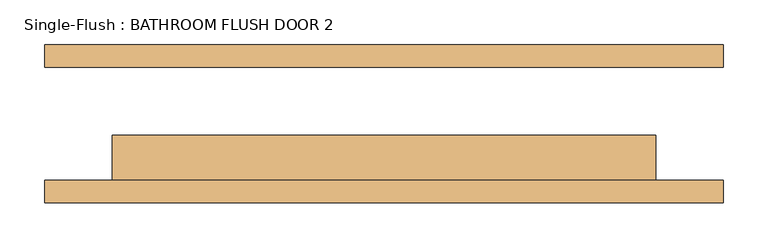
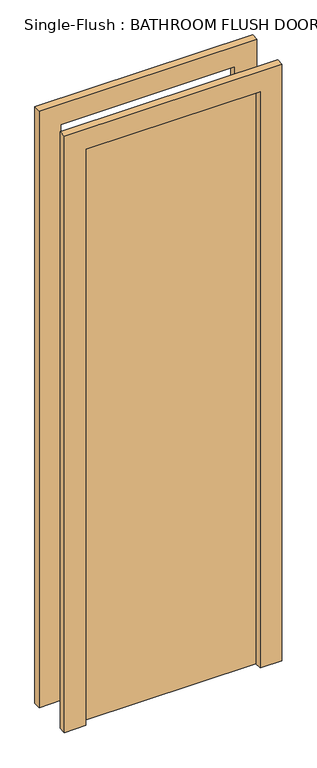
"""IFC4 building model written with IfcOpenShell, lengths in millimetres: door geometry, Single-Flush : BATHROOM FLUSH DOOR 2."""

from ifc_helpers import new_model, si_unit, frame, origin, origin_with_axes, place, context, project, spatial, polyline, outline, extrude, source, transform, mapped, element, save


def single_flush_bathroom_flush_door_2_931cabab(model_context):
    return source(origin(), model_context, "Body", "SweptSolid", [
        extrude(outline(polyline([(2209.8, -381.0), (0.0, -381.0), (0.0, -304.8), (2133.6, -304.8), (2133.6, 304.8), (0.0, 304.8), (0.0, 381.0), (2209.8, 381.0), (2209.8, -381.0)])), frame((0.0, -88.9, 0.0), z_axis=(0.0, 1.0, 0.0), x_axis=(0.0, 0.0, 1.0)), (0.0, 0.0, 1.0), 25.4),
        extrude(outline(polyline([(2209.8, 381.0), (2209.8, -381.0), (0.0, -381.0), (0.0, -304.8), (2133.6, -304.8), (2133.6, 304.8), (0.0, 304.8), (0.0, 381.0), (2209.8, 381.0)])), frame((0.0, 63.5, 0.0), z_axis=(0.0, 1.0, 0.0), x_axis=(0.0, 0.0, 1.0)), (0.0, 0.0, 1.0), 25.4),
        extrude(outline(polyline([(304.8, -12.7), (304.8, -63.5), (-304.8, -63.5), (-304.8, -12.7), (304.8, -12.7)])), origin_with_axes(), (0.0, 0.0, 1.0), 2133.6),
    ])


if __name__ == "__main__":
    model = new_model("IFC4")
    model_context = context("Model", 3, world=origin())
    ifc_project = project(units=[si_unit("LENGTHUNIT", "METRE", prefix="MILLI")], contexts=[model_context])
    site = spatial("IfcSite", under=ifc_project)
    building = spatial("IfcBuilding", under=site)
    placement = place(None, origin())
    single_flush_bathroom_flush_door_2_shape = single_flush_bathroom_flush_door_2_931cabab(model_context)
    element("IfcDoor", 1, ObjectType="Single-Flush : BATHROOM FLUSH DOOR 2", at=placement, inside=building, context=model_context, shape_type="MappedRepresentation", body=[
        mapped(single_flush_bathroom_flush_door_2_shape, transform((0.0, 0.0, 0.0), x_axis=(1.0, 0.0, 0.0), y_axis=(0.0, 1.0, 0.0), z_axis=(0.0, 0.0, 1.0))),
    ])
    save(model, "model.ifc")

# Revit data of these elements
# Type "Single-Flush : BATHROOM FLUSH DOOR 2"
#   Type Mark = "11"
#   Construction Type Id = "MDOOR"
#   Assembly Code = "C1020"
#   Analytic Construction = "Metal"
#   Thickness = 0' - 2"
#   Heat Transfer Coefficient (U) = 0.651978 BTU/(h·ft²·°F)
#   Height = 7' - 0"
#   Trim Projection Ext = 0' - 1"
#   Trim Projection Int = 0' - 1"
#   Trim Width = 0' - 3"
#   Width = 2' - 0"
#   Define Thermal Properties by = 1
#   Door Material = Door - Panel
#   Frame Material = Door - Frame
#   Visual Light Transmittance = 0
#   Solar Heat Gain Coefficient = 0
#   Function = (empty or 0)
#   Wall Closure = (empty or 0)
# Element 1 (IfcDoor, "Single-Flush : BATHROOM FLUSH DOOR 2")
#   Materials on its faces: "Door - Frame", "Door - Panel"
# Materials
#   "Door - Panel": class "Wood", colour RGB 210 159 95, transparency 0, Cost = 0
#   "Door - Frame": colour RGB 118 70 51, transparency 0, Cost = 0
